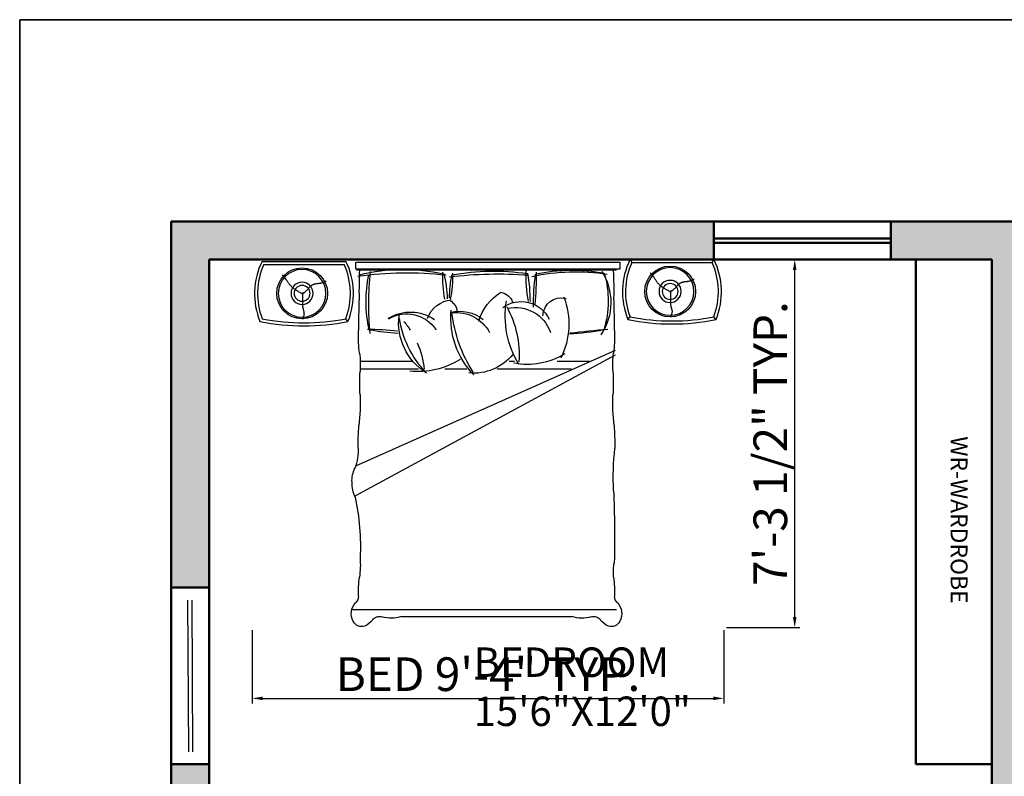
# Model space of a CAD drawing. Units: inches. Extents: x 1986 to 21484, y -1816 to 2016.
# Tile 44 of 85: x 2500 to 2734, y 1721 to 1901. Entities that reach past the tile are written whole.
import ezdxf

# ---------------------------------------------------------------- set-up
doc = ezdxf.new("R2010")
doc.units = ezdxf.units.IN
for name, color, linetype, lineweight in [('A-ANNO-DIMS', 2, 'Continuous', 18), ('A-ANNO-TEXT', 7, 'Continuous', 18), ('A-AREA-IDEN', 3, 'Continuous', 18), ('A-FURN', 8, 'Continuous', 18), ('A-GLAZ', 4, 'Continuous', 25), ('A-WALL', 7, 'Continuous', 50), ('A-WALL-PATT', 8, 'Continuous', 13), ('C-PROP', 7, 'Continuous', 35)]:
    doc.layers.add(name, color=color, linetype=linetype, lineweight=lineweight)
doc.layers.add('TEFRİŞ', color=11, linetype='Continuous')
doc.styles.get("Standard").update_dxf_attribs({"font": 'arial.ttf'})
doc.dimstyles.new('ISO-25', dxfattribs={"dimtxt": 8, "dimasz": 2.5, "dimexe": 1.25, "dimexo": 0.625, "dimtad": 1, "dimdec": 1, "dimlunit": 3, "dimtxsty": 'Standard', "dimcen": 2.5, "dimadec": 0, "dimazin": 0, "dimtfac": 1, "dimtdec": 1, "dimtmove": 0, "dimatfit": 3, "dimfxl": 1, "dimarcsym": 0})

# ---------------------------------------------------------------- blocks, each defined once
blk = doc.blocks.new('BED')
at = {"layer": 'TEFRİŞ'}
for p, q in [((2114.88, 1835.66), (2129.12, 1835.66)), ((2115.2, 1835.15), (2128.8, 1835.15)), ((2130.81, 1834.34), (2130.81, 1835.55)), ((2130.91, 1835.55), (2175.56, 1835.55)), ((2175.56, 1835.55), (2175.56, 1834.34)), ((2177.29, 1835.98), (2177.61, 1835.47)), ((2177.29, 1835.98), (2191.52, 1835.98)), ((2177.61, 1835.47), (2191.2, 1835.47)), ((2191.2, 1835.47), (2191.52, 1835.98)), ((2175.56, 1834.34), (2130.81, 1834.34)), ((2175, 1834.19), (2130.91, 1834.19)), ((2180.9, 1833.52), (2180.75, 1833.7)), ((2180.9, 1833.52), (2180.75, 1833.7)), ((2181.04, 1833.35), (2180.9, 1833.52)), ((2181.04, 1833.35), (2180.9, 1833.52)), ((2118.49, 1833.2), (2118.34, 1833.38)), ((2118.49, 1833.2), (2118.34, 1833.38)), ((2118.63, 1833.03), (2118.49, 1833.2)), ((2118.63, 1833.03), (2118.49, 1833.2)), ((2118.75, 1832.88), (2118.63, 1833.03)), ((2118.75, 1832.88), (2118.63, 1833.03)), ((2118.86, 1832.74), (2118.75, 1832.88)), ((2118.86, 1832.74), (2118.75, 1832.88)), ((2118.95, 1832.61), (2118.86, 1832.74)), ((2118.95, 1832.61), (2118.86, 1832.74)), ((2119.04, 1832.48), (2118.95, 1832.61)), ((2119.04, 1832.48), (2118.95, 1832.61)), ((2119.12, 1832.37), (2119.04, 1832.48)), ((2119.12, 1832.37), (2119.04, 1832.48)), ((2119.19, 1832.26), (2119.12, 1832.37)), ((2119.19, 1832.26), (2119.12, 1832.37)), ((2119.26, 1832.16), (2119.19, 1832.26)), ((2119.26, 1832.16), (2119.19, 1832.26)), ((2119.32, 1832.06), (2119.26, 1832.16)), ((2119.32, 1832.06), (2119.26, 1832.16)), ((2119.39, 1831.97), (2119.32, 1832.06)), ((2119.39, 1831.97), (2119.32, 1832.06)), ((2119.45, 1831.89), (2119.39, 1831.97)), ((2119.45, 1831.89), (2119.39, 1831.97)), ((2119.51, 1831.81), (2119.45, 1831.89)), ((2119.51, 1831.81), (2119.45, 1831.89)), ((2119.57, 1831.73), (2119.51, 1831.81)), ((2119.57, 1831.73), (2119.51, 1831.81)), ((2123.55, 1831.74), (2123.62, 1831.77)), ((2123.55, 1831.74), (2123.62, 1831.77)), ((2123.62, 1831.77), (2123.69, 1831.8)), ((2123.62, 1831.77), (2123.69, 1831.8)), ((2123.69, 1831.8), (2123.77, 1831.82)), ((2123.69, 1831.8), (2123.77, 1831.82)), ((2123.77, 1831.82), (2123.84, 1831.84)), ((2123.77, 1831.82), (2123.84, 1831.84)), ((2123.84, 1831.84), (2123.91, 1831.86)), ((2123.84, 1831.84), (2123.91, 1831.86)), ((2123.91, 1831.86), (2123.98, 1831.87)), ((2123.91, 1831.86), (2123.98, 1831.87)), ((2123.98, 1831.87), (2124.06, 1831.89)), ((2123.98, 1831.87), (2124.06, 1831.89)), ((2124.06, 1831.89), (2124.13, 1831.9)), ((2124.06, 1831.89), (2124.13, 1831.9)), ((2124.13, 1831.9), (2124.2, 1831.91)), ((2124.13, 1831.9), (2124.2, 1831.91)), ((2124.2, 1831.91), (2124.27, 1831.91)), ((2124.2, 1831.91), (2124.27, 1831.91)), ((2124.27, 1831.91), (2124.35, 1831.92)), ((2124.27, 1831.91), (2124.35, 1831.92)), ((2124.35, 1831.92), (2124.42, 1831.93)), ((2124.35, 1831.92), (2124.42, 1831.93)), ((2124.42, 1831.93), (2124.49, 1831.94)), ((2124.42, 1831.93), (2124.49, 1831.94)), ((2124.49, 1831.94), (2124.56, 1831.95)), ((2124.49, 1831.94), (2124.56, 1831.95)), ((2124.56, 1831.95), (2124.64, 1831.96)), ((2124.56, 1831.95), (2124.64, 1831.96)), ((2124.64, 1831.96), (2124.71, 1831.98)), ((2124.64, 1831.96), (2124.71, 1831.98)), ((2124.71, 1831.98), (2124.79, 1831.99)), ((2124.71, 1831.98), (2124.79, 1831.99)), ((2124.79, 1831.99), (2124.87, 1832.01)), ((2124.79, 1831.99), (2124.87, 1832.01)), ((2124.87, 1832.01), (2124.96, 1832.03)), ((2124.87, 1832.01), (2124.96, 1832.03)), ((2124.96, 1832.03), (2125.05, 1832.05)), ((2124.96, 1832.03), (2125.05, 1832.05)), ((2125.05, 1832.05), (2125.14, 1832.08)), ((2125.05, 1832.05), (2125.14, 1832.08)), ((2125.14, 1832.08), (2125.23, 1832.11)), ((2125.14, 1832.08), (2125.23, 1832.11)), ((2125.23, 1832.11), (2125.33, 1832.14)), ((2125.23, 1832.11), (2125.33, 1832.14)), ((2125.33, 1832.14), (2125.42, 1832.17)), ((2125.33, 1832.14), (2125.42, 1832.17)), ((2125.42, 1832.17), (2125.52, 1832.21)), ((2125.42, 1832.17), (2125.52, 1832.21)), ((2125.52, 1832.21), (2125.6, 1832.25)), ((2125.52, 1832.21), (2125.6, 1832.25)), ((2125.6, 1832.25), (2125.68, 1832.3)), ((2125.6, 1832.25), (2125.68, 1832.3)), ((2125.68, 1832.3), (2125.75, 1832.35)), ((2125.68, 1832.3), (2125.75, 1832.35)), ((2181.16, 1833.2), (2181.04, 1833.35)), ((2181.16, 1833.2), (2181.04, 1833.35)), ((2181.26, 1833.06), (2181.16, 1833.2)), ((2181.26, 1833.06), (2181.16, 1833.2)), ((2181.36, 1832.93), (2181.26, 1833.06)), ((2181.36, 1832.93), (2181.26, 1833.06)), ((2181.44, 1832.8), (2181.36, 1832.93)), ((2181.44, 1832.8), (2181.36, 1832.93)), ((2181.52, 1832.69), (2181.44, 1832.8)), ((2181.52, 1832.69), (2181.44, 1832.8)), ((2181.59, 1832.58), (2181.52, 1832.69)), ((2181.59, 1832.58), (2181.52, 1832.69)), ((2181.66, 1832.48), (2181.59, 1832.58)), ((2181.66, 1832.48), (2181.59, 1832.58)), ((2181.73, 1832.38), (2181.66, 1832.48)), ((2181.73, 1832.38), (2181.66, 1832.48)), ((2181.79, 1832.29), (2181.73, 1832.38)), ((2181.79, 1832.29), (2181.73, 1832.38)), ((2181.85, 1832.21), (2181.79, 1832.29)), ((2181.85, 1832.21), (2181.79, 1832.29)), ((2181.92, 1832.13), (2181.85, 1832.21)), ((2181.92, 1832.13), (2181.85, 1832.21)), ((2181.97, 1832.05), (2181.92, 1832.13)), ((2181.97, 1832.05), (2181.92, 1832.13)), ((2182.03, 1831.97), (2181.97, 1832.05)), ((2182.03, 1831.97), (2181.97, 1832.05)), ((2182.09, 1831.9), (2182.03, 1831.97)), ((2182.09, 1831.9), (2182.03, 1831.97)), ((2182.15, 1831.83), (2182.09, 1831.9)), ((2182.15, 1831.83), (2182.09, 1831.9)), ((2182.21, 1831.76), (2182.15, 1831.83)), ((2182.21, 1831.76), (2182.15, 1831.83)), ((2182.27, 1831.7), (2182.21, 1831.76)), ((2182.27, 1831.7), (2182.21, 1831.76)), ((2185.48, 1831.72), (2185.55, 1831.78)), ((2185.48, 1831.72), (2185.55, 1831.78)), ((2185.55, 1831.78), (2185.61, 1831.84)), ((2185.55, 1831.78), (2185.61, 1831.84)), ((2185.61, 1831.84), (2185.68, 1831.9)), ((2185.61, 1831.84), (2185.68, 1831.9)), ((2185.68, 1831.9), (2185.75, 1831.95)), ((2185.68, 1831.9), (2185.75, 1831.95)), ((2185.75, 1831.95), (2185.82, 1831.99)), ((2185.75, 1831.95), (2185.82, 1831.99)), ((2185.82, 1831.99), (2185.89, 1832.03)), ((2185.82, 1831.99), (2185.89, 1832.03)), ((2185.89, 1832.03), (2185.96, 1832.06)), ((2185.89, 1832.03), (2185.96, 1832.06)), ((2185.96, 1832.06), (2186.03, 1832.09)), ((2185.96, 1832.06), (2186.03, 1832.09)), ((2186.03, 1832.09), (2186.1, 1832.12)), ((2186.03, 1832.09), (2186.1, 1832.12)), ((2186.1, 1832.12), (2186.17, 1832.14)), ((2186.1, 1832.12), (2186.17, 1832.14)), ((2186.17, 1832.14), (2186.24, 1832.16)), ((2186.17, 1832.14), (2186.24, 1832.16)), ((2186.24, 1832.16), (2186.32, 1832.18)), ((2186.24, 1832.16), (2186.32, 1832.18)), ((2186.32, 1832.18), (2186.39, 1832.19)), ((2186.32, 1832.18), (2186.39, 1832.19)), ((2186.39, 1832.19), (2186.46, 1832.21)), ((2186.39, 1832.19), (2186.46, 1832.21)), ((2186.46, 1832.21), (2186.53, 1832.22)), ((2186.46, 1832.21), (2186.53, 1832.22)), ((2186.53, 1832.22), (2186.61, 1832.23)), ((2186.53, 1832.22), (2186.61, 1832.23)), ((2186.61, 1832.23), (2186.68, 1832.23)), ((2186.61, 1832.23), (2186.68, 1832.23)), ((2186.68, 1832.23), (2186.75, 1832.24)), ((2186.68, 1832.23), (2186.75, 1832.24)), ((2186.75, 1832.24), (2186.82, 1832.25)), ((2186.75, 1832.24), (2186.82, 1832.25)), ((2186.82, 1832.25), (2186.9, 1832.26)), ((2186.82, 1832.25), (2186.9, 1832.26)), ((2186.9, 1832.26), (2186.97, 1832.27)), ((2186.9, 1832.26), (2186.97, 1832.27)), ((2186.97, 1832.27), (2187.04, 1832.28)), ((2186.97, 1832.27), (2187.04, 1832.28)), ((2187.04, 1832.28), (2187.12, 1832.3)), ((2187.04, 1832.28), (2187.12, 1832.3)), ((2187.12, 1832.3), (2187.2, 1832.31)), ((2187.12, 1832.3), (2187.2, 1832.31)), ((2187.2, 1832.31), (2187.28, 1832.33)), ((2187.2, 1832.31), (2187.28, 1832.33)), ((2187.28, 1832.33), (2187.36, 1832.35)), ((2187.28, 1832.33), (2187.36, 1832.35)), ((2187.36, 1832.35), (2187.45, 1832.37)), ((2187.36, 1832.35), (2187.45, 1832.37)), ((2187.45, 1832.37), (2187.54, 1832.4)), ((2187.45, 1832.37), (2187.54, 1832.4)), ((2187.54, 1832.4), (2187.64, 1832.43)), ((2187.54, 1832.4), (2187.64, 1832.43)), ((2187.64, 1832.43), (2187.74, 1832.46)), ((2187.64, 1832.43), (2187.74, 1832.46)), ((2187.74, 1832.46), (2187.83, 1832.49)), ((2187.74, 1832.46), (2187.83, 1832.49)), ((2187.83, 1832.49), (2187.92, 1832.53)), ((2187.83, 1832.49), (2187.92, 1832.53)), ((2187.92, 1832.53), (2188.01, 1832.57)), ((2187.92, 1832.53), (2188.01, 1832.57)), ((2188.01, 1832.57), (2188.09, 1832.62)), ((2188.01, 1832.57), (2188.09, 1832.62)), ((2188.09, 1832.62), (2188.15, 1832.67)), ((2188.09, 1832.62), (2188.15, 1832.67)), ((2119.63, 1831.65), (2119.57, 1831.73)), ((2119.63, 1831.65), (2119.57, 1831.73)), ((2119.69, 1831.58), (2119.63, 1831.65)), ((2119.69, 1831.58), (2119.63, 1831.65)), ((2119.75, 1831.51), (2119.69, 1831.58)), ((2119.75, 1831.51), (2119.69, 1831.58)), ((2119.81, 1831.44), (2119.75, 1831.51)), ((2119.81, 1831.44), (2119.75, 1831.51)), ((2119.87, 1831.38), (2119.81, 1831.44)), ((2119.87, 1831.38), (2119.81, 1831.44)), ((2119.93, 1831.31), (2119.87, 1831.38)), ((2119.93, 1831.31), (2119.87, 1831.38)), ((2119.99, 1831.25), (2119.93, 1831.31)), ((2119.99, 1831.25), (2119.93, 1831.31)), ((2120.05, 1831.2), (2119.99, 1831.25)), ((2120.05, 1831.2), (2119.99, 1831.25)), ((2120.12, 1831.14), (2120.05, 1831.2)), ((2120.12, 1831.14), (2120.05, 1831.2)), ((2120.18, 1831.09), (2120.12, 1831.14)), ((2120.18, 1831.09), (2120.12, 1831.14)), ((2120.25, 1831.04), (2120.18, 1831.09)), ((2120.25, 1831.04), (2120.18, 1831.09)), ((2120.32, 1830.99), (2120.25, 1831.04)), ((2120.32, 1830.99), (2120.25, 1831.04)), ((2120.39, 1830.94), (2120.32, 1830.99)), ((2120.39, 1830.94), (2120.32, 1830.99)), ((2120.47, 1830.9), (2120.39, 1830.94)), ((2120.47, 1830.9), (2120.39, 1830.94)), ((2120.54, 1830.85), (2120.47, 1830.9)), ((2120.54, 1830.85), (2120.47, 1830.9)), ((2120.62, 1830.8), (2120.54, 1830.85)), ((2120.62, 1830.8), (2120.54, 1830.85)), ((2120.7, 1830.75), (2120.62, 1830.8)), ((2120.7, 1830.75), (2120.62, 1830.8)), ((2120.79, 1830.7), (2120.7, 1830.75)), ((2120.79, 1830.7), (2120.7, 1830.75)), ((2120.88, 1830.65), (2120.79, 1830.7)), ((2120.88, 1830.65), (2120.79, 1830.7)), ((2120.98, 1830.59), (2120.88, 1830.65)), ((2120.98, 1830.59), (2120.88, 1830.65)), ((2121.09, 1830.52), (2120.98, 1830.59)), ((2121.09, 1830.52), (2120.98, 1830.59)), ((2121.21, 1830.45), (2121.09, 1830.52)), ((2121.21, 1830.45), (2121.09, 1830.52)), ((2121.34, 1830.38), (2121.21, 1830.45)), ((2121.34, 1830.38), (2121.21, 1830.45)), ((2121.49, 1830.29), (2121.34, 1830.38)), ((2121.49, 1830.29), (2121.34, 1830.38)), ((2121.66, 1830.21), (2121.49, 1830.29)), ((2121.66, 1830.21), (2121.49, 1830.29)), ((2121.66, 1830.18), (2121.87, 1830.29)), ((2121.66, 1830.18), (2121.87, 1830.29)), ((2121.85, 1830.11), (2121.66, 1830.21)), ((2121.85, 1830.11), (2121.66, 1830.21)), ((2121.76, 1830.38), (2121.74, 1830.17)), ((2121.76, 1830.38), (2121.74, 1830.17)), ((2121.74, 1830.17), (2121.74, 1829.99)), ((2121.74, 1830.17), (2121.74, 1829.99)), ((2121.87, 1830.29), (2122.04, 1830.4)), ((2121.87, 1830.29), (2122.04, 1830.4)), ((2122.04, 1830.4), (2122.2, 1830.51)), ((2122.04, 1830.4), (2122.2, 1830.51)), ((2122.2, 1830.51), (2122.33, 1830.61)), ((2122.2, 1830.51), (2122.33, 1830.61)), ((2122.33, 1830.61), (2122.45, 1830.72)), ((2122.33, 1830.61), (2122.45, 1830.72)), ((2122.45, 1830.72), (2122.55, 1830.82)), ((2122.45, 1830.72), (2122.55, 1830.82)), ((2122.55, 1830.82), (2122.64, 1830.91)), ((2122.55, 1830.82), (2122.64, 1830.91)), ((2122.64, 1830.91), (2122.72, 1831.01)), ((2122.64, 1830.91), (2122.72, 1831.01)), ((2122.72, 1831.01), (2122.8, 1831.09)), ((2122.72, 1831.01), (2122.8, 1831.09)), ((2122.8, 1831.09), (2122.87, 1831.18)), ((2122.8, 1831.09), (2122.87, 1831.18)), ((2122.87, 1831.18), (2122.94, 1831.26)), ((2122.87, 1831.18), (2122.94, 1831.26)), ((2122.94, 1831.26), (2123.01, 1831.33)), ((2122.94, 1831.26), (2123.01, 1831.33)), ((2123.01, 1831.33), (2123.08, 1831.4)), ((2123.01, 1831.33), (2123.08, 1831.4)), ((2123.08, 1831.4), (2123.14, 1831.46)), ((2123.08, 1831.4), (2123.14, 1831.46)), ((2123.14, 1831.46), (2123.21, 1831.52)), ((2123.14, 1831.46), (2123.21, 1831.52)), ((2123.21, 1831.52), (2123.27, 1831.58)), ((2123.21, 1831.52), (2123.27, 1831.58)), ((2123.27, 1831.58), (2123.34, 1831.63)), ((2123.27, 1831.58), (2123.34, 1831.63)), ((2123.34, 1831.63), (2123.41, 1831.67)), ((2123.34, 1831.63), (2123.41, 1831.67)), ((2123.41, 1831.67), (2123.48, 1831.71)), ((2123.41, 1831.67), (2123.48, 1831.71)), ((2123.48, 1831.71), (2123.55, 1831.74)), ((2123.48, 1831.71), (2123.55, 1831.74)), ((2182.33, 1831.63), (2182.27, 1831.7)), ((2182.33, 1831.63), (2182.27, 1831.7)), ((2182.4, 1831.57), (2182.33, 1831.63)), ((2182.4, 1831.57), (2182.33, 1831.63)), ((2182.46, 1831.52), (2182.4, 1831.57)), ((2182.46, 1831.52), (2182.4, 1831.57)), ((2182.52, 1831.46), (2182.46, 1831.52)), ((2182.52, 1831.46), (2182.46, 1831.52)), ((2182.59, 1831.41), (2182.52, 1831.46)), ((2182.59, 1831.41), (2182.52, 1831.46)), ((2182.66, 1831.36), (2182.59, 1831.41)), ((2182.66, 1831.36), (2182.59, 1831.41)), ((2182.73, 1831.31), (2182.66, 1831.36)), ((2182.73, 1831.31), (2182.66, 1831.36)), ((2182.8, 1831.26), (2182.73, 1831.31)), ((2182.8, 1831.26), (2182.73, 1831.31)), ((2182.87, 1831.22), (2182.8, 1831.26)), ((2182.87, 1831.22), (2182.8, 1831.26)), ((2182.95, 1831.17), (2182.87, 1831.22)), ((2182.95, 1831.17), (2182.87, 1831.22)), ((2183.03, 1831.12), (2182.95, 1831.17)), ((2183.03, 1831.12), (2182.95, 1831.17)), ((2183.11, 1831.07), (2183.03, 1831.12)), ((2183.11, 1831.07), (2183.03, 1831.12)), ((2183.2, 1831.02), (2183.11, 1831.07)), ((2183.2, 1831.02), (2183.11, 1831.07)), ((2183.29, 1830.97), (2183.2, 1831.02)), ((2183.29, 1830.97), (2183.2, 1831.02)), ((2183.39, 1830.91), (2183.29, 1830.97)), ((2183.39, 1830.91), (2183.29, 1830.97)), ((2183.49, 1830.84), (2183.39, 1830.91)), ((2183.49, 1830.84), (2183.39, 1830.91)), ((2183.61, 1830.77), (2183.49, 1830.84)), ((2183.61, 1830.77), (2183.49, 1830.84)), ((2183.75, 1830.7), (2183.61, 1830.77)), ((2183.75, 1830.7), (2183.61, 1830.77)), ((2183.9, 1830.61), (2183.75, 1830.7)), ((2183.9, 1830.61), (2183.75, 1830.7)), ((2184.06, 1830.53), (2183.9, 1830.61)), ((2184.06, 1830.53), (2183.9, 1830.61)), ((2184.25, 1830.43), (2184.06, 1830.53)), ((2184.25, 1830.43), (2184.06, 1830.53)), ((2184.07, 1830.5), (2184.27, 1830.61)), ((2184.07, 1830.5), (2184.27, 1830.61)), ((2184.15, 1830.49), (2184.14, 1830.31)), ((2184.15, 1830.49), (2184.14, 1830.31)), ((2184.14, 1830.31), (2184.14, 1830.15)), ((2184.14, 1830.31), (2184.14, 1830.15)), ((2184.14, 1830.15), (2184.14, 1830.01)), ((2184.14, 1830.15), (2184.14, 1830.01)), ((2184.17, 1830.7), (2184.15, 1830.49)), ((2184.17, 1830.7), (2184.15, 1830.49)), ((2184.27, 1830.61), (2184.45, 1830.72)), ((2184.27, 1830.61), (2184.45, 1830.72)), ((2184.45, 1830.72), (2184.6, 1830.83)), ((2184.45, 1830.72), (2184.6, 1830.83)), ((2184.6, 1830.83), (2184.74, 1830.93)), ((2184.6, 1830.83), (2184.74, 1830.93)), ((2184.74, 1830.93), (2184.85, 1831.04)), ((2184.74, 1830.93), (2184.85, 1831.04)), ((2184.85, 1831.04), (2184.95, 1831.14)), ((2184.85, 1831.04), (2184.95, 1831.14)), ((2184.95, 1831.14), (2185.05, 1831.23)), ((2184.95, 1831.14), (2185.05, 1831.23)), ((2185.05, 1831.23), (2185.13, 1831.33)), ((2185.05, 1831.23), (2185.13, 1831.33)), ((2185.13, 1831.33), (2185.21, 1831.41)), ((2185.13, 1831.33), (2185.21, 1831.41)), ((2185.21, 1831.41), (2185.28, 1831.5)), ((2185.21, 1831.41), (2185.28, 1831.5)), ((2185.28, 1831.5), (2185.35, 1831.58)), ((2185.28, 1831.5), (2185.35, 1831.58)), ((2185.35, 1831.58), (2185.42, 1831.65)), ((2185.35, 1831.58), (2185.42, 1831.65)), ((2185.42, 1831.65), (2185.48, 1831.72)), ((2185.42, 1831.65), (2185.48, 1831.72)), ((2121.74, 1829.99), (2121.73, 1829.83)), ((2121.74, 1829.99), (2121.73, 1829.83)), ((2121.73, 1829.83), (2121.73, 1829.69)), ((2121.73, 1829.83), (2121.73, 1829.69)), ((2121.73, 1829.69), (2121.73, 1829.57)), ((2121.73, 1829.69), (2121.73, 1829.57)), ((2121.73, 1829.57), (2121.73, 1829.45)), ((2121.73, 1829.57), (2121.73, 1829.45)), ((2121.73, 1829.45), (2121.74, 1829.35)), ((2121.73, 1829.45), (2121.74, 1829.35)), ((2121.74, 1828.89), (2121.73, 1828.8)), ((2121.74, 1828.89), (2121.73, 1828.8)), ((2121.73, 1828.8), (2121.73, 1828.72)), ((2121.73, 1828.8), (2121.73, 1828.72)), ((2121.73, 1828.72), (2121.73, 1828.64)), ((2121.73, 1828.72), (2121.73, 1828.64)), ((2121.73, 1828.64), (2121.73, 1828.56)), ((2121.73, 1828.64), (2121.73, 1828.56)), ((2121.73, 1828.56), (2121.73, 1828.48)), ((2121.73, 1828.56), (2121.73, 1828.48)), ((2121.73, 1828.48), (2121.73, 1828.4)), ((2121.73, 1828.48), (2121.73, 1828.4)), ((2121.74, 1829.35), (2121.74, 1829.25)), ((2121.74, 1829.35), (2121.74, 1829.25)), ((2121.74, 1829.25), (2121.74, 1829.16)), ((2121.74, 1829.25), (2121.74, 1829.16)), ((2121.74, 1829.16), (2121.74, 1829.06)), ((2121.74, 1829.16), (2121.74, 1829.06)), ((2121.74, 1829.06), (2121.74, 1828.97)), ((2121.74, 1829.06), (2121.74, 1828.97)), ((2121.74, 1828.97), (2121.74, 1828.89)), ((2121.74, 1828.97), (2121.74, 1828.89)), ((2184.14, 1829.04), (2184.13, 1828.96)), ((2184.14, 1829.04), (2184.13, 1828.96)), ((2184.13, 1828.96), (2184.13, 1828.88)), ((2184.13, 1828.96), (2184.13, 1828.88)), ((2184.13, 1828.88), (2184.13, 1828.8)), ((2184.13, 1828.88), (2184.13, 1828.8)), ((2184.13, 1828.8), (2184.14, 1828.72)), ((2184.13, 1828.8), (2184.14, 1828.72)), ((2184.14, 1830.01), (2184.14, 1829.89)), ((2184.14, 1830.01), (2184.14, 1829.89)), ((2184.14, 1829.89), (2184.14, 1829.77)), ((2184.14, 1829.89), (2184.14, 1829.77)), ((2184.14, 1829.77), (2184.14, 1829.67)), ((2184.14, 1829.77), (2184.14, 1829.67)), ((2184.14, 1829.67), (2184.15, 1829.57)), ((2184.14, 1829.67), (2184.15, 1829.57)), ((2184.15, 1829.38), (2184.14, 1829.29)), ((2184.15, 1829.38), (2184.14, 1829.29)), ((2184.14, 1829.29), (2184.14, 1829.21)), ((2184.14, 1829.29), (2184.14, 1829.21)), ((2184.14, 1829.21), (2184.14, 1829.12)), ((2184.14, 1829.21), (2184.14, 1829.12)), ((2184.14, 1829.12), (2184.14, 1829.04)), ((2184.14, 1829.12), (2184.14, 1829.04)), ((2184.14, 1828.72), (2184.14, 1828.65)), ((2184.14, 1828.72), (2184.14, 1828.65)), ((2184.14, 1828.65), (2184.15, 1828.57)), ((2184.14, 1828.65), (2184.15, 1828.57)), ((2184.15, 1829.57), (2184.15, 1829.48)), ((2184.15, 1829.57), (2184.15, 1829.48)), ((2184.15, 1829.48), (2184.15, 1829.38)), ((2184.15, 1829.48), (2184.15, 1829.38)), ((2184.15, 1828.57), (2184.15, 1828.5)), ((2184.15, 1828.57), (2184.15, 1828.5)), ((2184.15, 1828.5), (2184.16, 1828.42)), ((2184.15, 1828.5), (2184.16, 1828.42)), ((2184.16, 1828.42), (2184.17, 1828.35)), ((2184.16, 1828.42), (2184.17, 1828.35)), ((2121.73, 1828.4), (2121.73, 1828.33)), ((2121.73, 1828.4), (2121.73, 1828.33)), ((2121.73, 1828.33), (2121.74, 1828.25)), ((2121.73, 1828.33), (2121.74, 1828.25)), ((2121.74, 1828.25), (2121.75, 1828.18)), ((2121.74, 1828.25), (2121.75, 1828.18)), ((2121.75, 1828.18), (2121.75, 1828.1)), ((2121.75, 1828.18), (2121.75, 1828.1)), ((2121.75, 1828.1), (2121.76, 1828.03)), ((2121.75, 1828.1), (2121.76, 1828.03)), ((2121.76, 1828.03), (2121.78, 1827.95)), ((2121.76, 1828.03), (2121.78, 1827.95)), ((2121.78, 1827.95), (2121.79, 1827.88)), ((2121.78, 1827.95), (2121.79, 1827.88)), ((2121.79, 1827.88), (2121.8, 1827.8)), ((2121.79, 1827.88), (2121.8, 1827.8)), ((2121.8, 1827.8), (2121.82, 1827.72)), ((2121.8, 1827.8), (2121.82, 1827.72)), ((2121.82, 1827.72), (2121.84, 1827.65)), ((2121.82, 1827.72), (2121.84, 1827.65)), ((2121.84, 1827.65), (2121.85, 1827.57)), ((2121.84, 1827.65), (2121.85, 1827.57)), ((2121.85, 1827.57), (2121.87, 1827.49)), ((2121.85, 1827.57), (2121.87, 1827.49)), ((2121.87, 1827.49), (2121.89, 1827.41)), ((2121.87, 1827.49), (2121.89, 1827.41)), ((2121.89, 1827.41), (2121.91, 1827.33)), ((2121.89, 1827.41), (2121.91, 1827.33)), ((2121.91, 1827.33), (2121.93, 1827.26)), ((2121.91, 1827.33), (2121.93, 1827.26)), ((2121.93, 1827.26), (2121.95, 1827.18)), ((2121.93, 1827.26), (2121.95, 1827.18)), ((2121.95, 1827.18), (2121.97, 1827.09)), ((2121.95, 1827.18), (2121.97, 1827.09)), ((2121.97, 1827.09), (2121.99, 1827.01)), ((2121.97, 1827.09), (2121.99, 1827.01)), ((2121.99, 1827.01), (2122, 1826.93)), ((2121.99, 1827.01), (2122, 1826.93)), ((2122, 1826.74), (2121.99, 1826.64)), ((2122, 1826.74), (2121.99, 1826.64)), ((2122, 1826.93), (2122.01, 1826.84)), ((2122, 1826.93), (2122.01, 1826.84)), ((2122.01, 1826.84), (2122, 1826.74)), ((2122.01, 1826.84), (2122, 1826.74)), ((2184.17, 1828.35), (2184.18, 1828.27)), ((2184.17, 1828.35), (2184.18, 1828.27)), ((2184.18, 1828.27), (2184.19, 1828.2)), ((2184.18, 1828.27), (2184.19, 1828.2)), ((2184.19, 1828.2), (2184.21, 1828.12)), ((2184.19, 1828.2), (2184.21, 1828.12)), ((2184.21, 1828.12), (2184.22, 1828.04)), ((2184.21, 1828.12), (2184.22, 1828.04)), ((2184.22, 1828.04), (2184.24, 1827.97)), ((2184.22, 1828.04), (2184.24, 1827.97)), ((2184.24, 1827.97), (2184.26, 1827.89)), ((2184.24, 1827.97), (2184.26, 1827.89)), ((2184.26, 1827.89), (2184.28, 1827.81)), ((2184.26, 1827.89), (2184.28, 1827.81)), ((2184.28, 1827.81), (2184.3, 1827.73)), ((2184.28, 1827.81), (2184.3, 1827.73)), ((2184.3, 1827.73), (2184.32, 1827.65)), ((2184.3, 1827.73), (2184.32, 1827.65)), ((2184.32, 1827.65), (2184.34, 1827.58)), ((2184.32, 1827.65), (2184.34, 1827.58)), ((2184.35, 1826.74), (2184.32, 1826.63)), ((2184.35, 1826.74), (2184.32, 1826.63)), ((2184.34, 1827.58), (2184.36, 1827.5)), ((2184.34, 1827.58), (2184.36, 1827.5)), ((2184.38, 1826.86), (2184.35, 1826.74)), ((2184.38, 1826.86), (2184.35, 1826.74)), ((2184.36, 1827.5), (2184.38, 1827.41)), ((2184.36, 1827.5), (2184.38, 1827.41)), ((2184.38, 1827.41), (2184.4, 1827.33)), ((2184.38, 1827.41), (2184.4, 1827.33)), ((2184.4, 1826.96), (2184.38, 1826.86)), ((2184.4, 1826.96), (2184.38, 1826.86)), ((2184.4, 1827.33), (2184.41, 1827.25)), ((2184.4, 1827.33), (2184.41, 1827.25)), ((2184.41, 1827.06), (2184.4, 1826.96)), ((2184.41, 1827.06), (2184.4, 1826.96)), ((2184.41, 1827.25), (2184.41, 1827.16)), ((2184.41, 1827.25), (2184.41, 1827.16)), ((2184.41, 1827.16), (2184.41, 1827.06)), ((2184.41, 1827.16), (2184.41, 1827.06)), ((2121.78, 1825.93), (2121.74, 1825.8)), ((2121.78, 1825.93), (2121.74, 1825.8)), ((2121.83, 1826.06), (2121.78, 1825.93)), ((2121.83, 1826.06), (2121.78, 1825.93)), ((2121.87, 1826.19), (2121.83, 1826.06)), ((2121.87, 1826.19), (2121.83, 1826.06)), ((2121.91, 1826.31), (2121.87, 1826.19)), ((2121.91, 1826.31), (2121.87, 1826.19)), ((2121.95, 1826.42), (2121.91, 1826.31)), ((2121.95, 1826.42), (2121.91, 1826.31)), ((2121.97, 1826.54), (2121.95, 1826.42)), ((2121.97, 1826.54), (2121.95, 1826.42)), ((2121.99, 1826.64), (2121.97, 1826.54)), ((2121.99, 1826.64), (2121.97, 1826.54)), ((2129.46, 1825.49), (2129.09, 1825.93)), ((2176.94, 1825.81), (2177.31, 1826.25)), ((2184.19, 1826.25), (2184.14, 1826.12)), ((2184.19, 1826.25), (2184.14, 1826.12)), ((2184.23, 1826.38), (2184.19, 1826.25)), ((2184.23, 1826.38), (2184.19, 1826.25)), ((2184.28, 1826.51), (2184.23, 1826.38)), ((2184.28, 1826.51), (2184.23, 1826.38)), ((2184.32, 1826.63), (2184.28, 1826.51)), ((2184.32, 1826.63), (2184.28, 1826.51)), ((2191.87, 1825.81), (2191.5, 1826.25)), ((2174.77, 1820.53), (2130.76, 1800.91)), ((2174.77, 1819.77), (2130.6, 1795.83)), ((2140.43, 1818.69), (2131.53, 1818.69)), ((2157.71, 1818.69), (2156.77, 1818.69)), ((2170.41, 1818.69), (2164.92, 1818.69)), ((2141.43, 1817.4), (2131.53, 1817.4)), ((2149.62, 1817.4), (2145.88, 1817.4)), ((2167.36, 1817.4), (2154.77, 1817.4)), ((2175, 1776.57), (2130.11, 1776.57)), ((2138.52, 1775.41), (2167.39, 1775.41))]:
    blk.add_line(p, q, dxfattribs=at)
for centre, radius, start, end in [((2126, 1830.19), 12.39, 153.8162, 202.314), ((2126, 1830.19), 11.88, 155.3335, 201.0157), ((2118, 1830.19), 11.88, 338.9843, 24.6665), ((2118, 1830.19), 12.39, 337.686, 26.1838), ((2188.4, 1830.51), 12.39, 153.8162, 202.314), ((2188.4, 1830.51), 11.88, 155.3335, 201.0157), ((2180.41, 1830.51), 11.88, 338.9843, 24.6665), ((2180.41, 1830.51), 12.39, 337.686, 26.1838), ((2122, 1861.35), 36.63, 258.2443, 281.7557), ((2122, 1861.35), 36.12, 258.6773, 281.3227), ((2184.41, 1861.67), 36.63, 258.2443, 281.7557), ((2184.41, 1861.67), 36.12, 258.6773, 281.3227)]:
    blk.add_arc(centre, radius, start, end, dxfattribs=at)
at = {"layer": 'TEFRİŞ', "extrusion": (0, 0, -1)}
for centre, major_axis, ratio, start_param, end_param in [((2121.68, 1830.24), (-3.05, -3.05), 1, 3.926991, 10.210176), ((2121.68, 1830.24), (2.86, -2.86), 1, 5.497787, 11.780972), ((2121.68, 1830.24), (2.86, -2.86), 1, 5.497787, 11.780972), ((2139.43, 1773.84), (-42.35, 42.35), 1, 0.646251, 0.896949), ((2206.14, 1830.73), (-52.86, -52.86), 1, 0.767743, 0.83177), ((2138.85, 1803.05), (-22.1, 22.1), 1, 0.544604, 1.006234), ((2181.61, 1828.44), (-34.39, 34.39), 1, -0.888486, -0.672463), ((2164.51, 1832.79), (-13.41, 13.41), 1, -0.974476, -0.730892), ((2127.6, 1828.81), (-13.23, 13.23), 1, 2.100388, 2.328052), ((2155, 1761.9), (-50.65, -50.65), 1, 2.239512, 2.426533), ((2128.44, 1832.96), (-13.26, -13.26), 1, 3.889049, 4.127298), ((2154.12, 1796.61), (-26.46, 26.46), 1, 0.596409, 0.940188), ((2183.72, 1833.22), (-17, 17), 1, -0.967105, -0.749712), ((2134, 1828.8), (-18.62, 18.62), 1, 2.173461, 2.355043), ((2168.35, 1789.27), (-1.33, 44.62), 0.875277, -0.163954, 0.163954), ((2199.2, 1828.45), (-27.06, -27.06), 1, 0.770625, 0.917228), ((2087.32, 1833.96), (-52.37, 52.37), 1, 2.358049, 2.431787), ((2167.6, 1797.72), (-0.51, 36.47), 0.865194, -0.185965, 0.185965), ((2164.15, 1828.7), (-6.99, 6.99), 1, 1.789136, 2.946702), ((2156.76, 1828.98), (-11.9, -11.9), 1, 3.646453, 4.226155), ((2099.77, 1830.73), (-52.86, 52.86), 1, 2.311571, 2.373849), ((2184.09, 1830.56), (-3.05, -3.05), 1, 3.926991, 10.210176), ((2184.09, 1830.56), (2.86, -2.86), 1, 5.497787, 11.780972), ((2184.09, 1830.56), (2.86, -2.86), 1, 5.497787, 11.780972), ((2121.68, 1830.24), (1.33, -1.33), 1, 5.497787, 11.780972), ((2121.68, 1830.24), (1.33, -1.33), 1, 5.497787, 11.780972), ((2154.7, 1828.89), (-15.68, 15.68), 1, -1.00675, -0.580436), ((2172.01, 1828.66), (-17.93, 17.93), 1, -0.753394, -0.598744), ((2184.09, 1830.56), (1.33, -1.33), 1, 5.497787, 11.780972), ((2184.09, 1830.56), (1.33, -1.33), 1, 5.497787, 11.780972), ((2184.09, 1830.56), (0.952, -0.952), 1, 5.497787, 11.780972), ((2184.09, 1830.56), (0.952, -0.952), 1, 5.497787, 11.780972), ((2121.68, 1830.24), (0.952, -0.952), 1, 5.497787, 11.780972), ((2121.68, 1830.24), (0.952, -0.952), 1, 5.497787, 11.780972), ((2159.55, 1823.33), (-5.81, 5.81), 1, -0.516587, 0.256776), ((2154.84, 1827.75), (-1.93, 1.93), 1, 0.997904, 1.977819), ((2675.38, 1815.09), (-384.79, -384.79), 1, 0.80103, 0.811711), ((2147.44, 1824.41), (-3.36, -3.36), 1, 1.11934, 2.270556), ((2145.66, 1827.01), (-1.62, 1.62), 1, 1.310976, 2.284591), ((2172, 1826.44), (-11.23, 11.23), 1, -1.332486, -0.624868), ((2158.82, 1823.55), (-3.74, -3.74), 1, 1.730792, 3.47045), ((2166.67, 1824.96), (-2.93, 3.91), 0.760601, -0.723751, 0.723751), ((2153.88, 1825.05), (-9.22, 9.22), 1, 1.994956, 2.818753), ((1630.53, 1815.09), (-384.79, 384.79), 1, 2.329881, 2.340562), ((2140.05, 1819.86), (-5.1, 5.1), 1, 0.238357, 1.390139), ((2139.42, 1820.79), (-4.21, -4.21), 1, 1.82161, 3.349145), ((2160.6, 1825.98), (-9.68, -9.68), 1, 0.009196, 0.886853), ((2148.35, 1820.65), (-4.63, -4.63), 1, 2.117602, 3.020837), ((2147.86, 1820.64), (-4.48, 4.48), 1, 0.665914, 1.867503), ((2170.68, 1829.67), (-16.79, 16.79), 1, -1.354718, -0.902276), ((2141.71, 1819.83), (-11.86, 11.86), 1, 1.850844, 2.42862), ((2157.83, 1821.53), (-4.47, 4.47), 1, 0.576679, 2.021689), ((2148.15, 1825.25), (-7.14, -7.14), 1, 6.061986, 7.190757), ((2154.93, 1828.48), (-11.96, 11.96), 1, -1.530302, -0.934407), ((2127.37, 1815.76), (-10.68, 10.68), 1, 1.657204, 1.779381), ((2146.08, 1822.57), (-10.5, 10.5), 1, -0.951783, -0.716225), ((2132.43, 1774.09), (-35.41, -35.41), 1, 2.362911, 2.464592), ((2140.17, 1862.96), (-27.99, 27.99), 1, 3.983025, 4.107469), ((2165.73, 1860.69), (-26.41, -26.41), 1, 5.306413, 5.463767), ((2199.62, 1529.47), (-209.2, 209.2), 1, 0.675361, 0.697001), ((2159.82, 1822.57), (-10.5, -10.5), 1, 3.857817, 4.093375), ((2127.37, 1815.76), (-10.68, 10.68), 1, 1.94252, 2.248924), ((2111.06, 1818.12), (-14.48, 14.48), 1, 2.258605, 2.412359), ((2194.85, 1818.12), (-14.48, 14.48), 1, -0.841563, -0.687809), ((2141.33, 1830.48), (-9.55, -9.55), 1, 4.941413, 5.601673), ((2150.79, 1825.18), (-6, 6), 1, 3.032122, 4.026148), ((2159.02, 1834.9), (-3.04, 16.53), 0.830169, 2.822117, 3.461068), ((2169.92, 1815.01), (-27.2, -27.2), 1, 0.734393, 0.836404), ((2135.98, 1815.01), (-27.2, -27.2), 1, 3.875985, 3.977996), ((2098.24, 1811.68), (-23.54, -23.54), 1, 3.885834, 4.043401), ((2207.66, 1811.68), (-23.54, -23.54), 1, 0.668988, 0.826555), ((2189.03, 1803.74), (-40.91, -40.91), 1, 0.789771, 0.855756), ((2116.87, 1803.74), (-40.91, 40.91), 1, 2.285836, 2.351822), ((2122.14, 1803.63), (-6.39, -6.39), 1, 3.886359, 4.265474), ((2222.76, 1798.77), (-34.16, -34.16), 1, 0.743488, 0.893627), ((2135.02, 1798.41), (-3.45, 3.45), 1, -0.831635, -0.314979), ((2135.48, 1798), (-3.77, -3.77), 1, 0.329385, 0.820948), ((2148.06, 1790.38), (-0.75, 67.37), 0.394952, 1.480524, 1.661068), ((2127.76, 1790.23), (-1, 12.37), 0.296708, 1.141067, 2.000525), ((2118.49, 1784.2), (-9.24, -9.24), 1, 3.839645, 4.088086), ((2182.27, 1782.99), (-5.52, -5.52), 1, 0.671703, 0.993321), ((2162.12, 1778.86), (-21.85, 21.85), 1, -0.78611, -0.680117), ((2143.78, 1778.86), (-21.85, 21.85), 1, 2.250913, 2.356906), ((2129.83, 1778.8), (-0.986, 0.986), 1, 2.330985, 3.163296), ((2176.08, 1778.8), (-0.986, 0.986), 1, 4.690686, 5.522997), ((2132.72, 1775.92), (-1.91, -1.91), 1, 0.284117, 1.557111), ((2173.18, 1775.92), (-1.91, -1.91), 1, 3.155278, 4.428271), ((2134.73, 1774.06), (-0.964, -0.964), 1, 1.381176, 2.701227), ((2136.75, 1781.14), (-4.24, 4.24), 1, 3.62713, 4.188813), ((2169.16, 1781.14), (-4.24, 4.24), 1, 3.665169, 4.226852), ((2171.17, 1774.06), (-0.964, -0.964), 1, 2.011162, 3.331212), ((2131.79, 1775.28), (-1.11, 1.11), 1, 3.629269, 5.067473), ((2130.83, 1777), (-2.49, -2.49), 1, 4.590984, 5.084038), ((2175.07, 1777), (-2.49, 2.49), 1, 4.34074, 4.833793), ((2174.12, 1775.28), (-1.11, 1.11), 1, 2.786508, 4.224712)]:
    blk.add_ellipse(centre, major_axis=major_axis, ratio=ratio, start_param=start_param, end_param=end_param, dxfattribs=at)
blk = doc.blocks.new('WIN-36')
for p, q in [((0, 36), (0, 0)), ((0, 36), (0, 0)), ((1, 36), (1, 0))]:
    blk.add_line(p, q)
blk = doc.blocks.new('*D85')
at = {"layer": 'A-ANNO-DIMS', "color": 0, "lineweight": -2, "transparency": 16777216}
for p, q in [((2555.53, 1755.63), (2555.53, 1738.18)), ((2667.68, 1755.63), (2667.68, 1738.18)), ((2558.03, 1739.43), (2665.18, 1739.43))]:
    blk.add_line(p, q, dxfattribs=at)
at = {"layer": 'A-ANNO-DIMS', "color": 0, "transparency": 16777216}
for points in [[(2558.03, 1739.85), (2558.03, 1739.02), (2555.53, 1739.43)], [(2665.18, 1739.85), (2665.18, 1739.02), (2667.68, 1739.43)]]:
    blk.add_solid(points, dxfattribs=at)
at = {"layer": 'Defpoints', "color": 0, "transparency": 16777216}
for p in [(2555.53, 1756.26), (2667.68, 1756.26), (2667.68, 1739.43)]:
    blk.add_point(p, dxfattribs=at)
at = {"layer": 'A-ANNO-DIMS', "color": 0, "transparency": 16777216, "insert": (2611.6, 1744.14), "char_height": 8, "attachment_point": 5}
blk.add_mtext('BED 9\'-4" TYP.', dxfattribs=at)
blk = doc.blocks.new('*D86')
at = {"layer": 'A-ANNO-DIMS', "color": 0, "lineweight": -2, "transparency": 16777216}
for p, q in [((2668.3, 1843.75), (2685.75, 1843.75)), ((2684.5, 1758.76), (2684.5, 1841.25)), ((2668.3, 1756.26), (2685.75, 1756.26))]:
    blk.add_line(p, q, dxfattribs=at)
at = {"layer": 'A-ANNO-DIMS', "color": 0, "transparency": 16777216}
for points in [[(2684.08, 1841.25), (2684.91, 1841.25), (2684.5, 1843.75)], [(2684.08, 1758.76), (2684.91, 1758.76), (2684.5, 1756.26)]]:
    blk.add_solid(points, dxfattribs=at)
at = {"layer": 'Defpoints', "color": 0, "transparency": 16777216}
for p in [(2667.68, 1843.75), (2684.5, 1843.75), (2667.68, 1756.26)]:
    blk.add_point(p, dxfattribs=at)
at = {"layer": 'A-ANNO-DIMS', "color": 0, "transparency": 16777216, "insert": (2679.73, 1800), "char_height": 8, "attachment_point": 5, "rotation": 90}
blk.add_mtext('7\'-3 1/2" TYP.', dxfattribs=at)

msp = doc.modelspace()

# ---------------------------------------------------------------- hatches: boundary and pattern name
at = {"layer": 'A-WALL-PATT'}
h = msp.add_hatch(color=256, dxfattribs=at)
h.dxf.hatch_style = 1
h.paths.add_polyline_path([(2545.31, 1843.75), (2665.31, 1843.75), (2665.31, 1852.75), (2536.31, 1852.75), (2536.31, 1765.75), (2545.31, 1765.75)])
h.paths.add_polyline_path([(2545.31, 1723.75), (2536.31, 1723.75), (2536.31, 1675.75), (2545.31, 1675.75), (2545.31, 1693.75), (2629.31, 1693.75), (2629.31, 1681.75), (2635.31, 1681.75), (2635.31, 1693.75), (2641.31, 1693.75), (2641.31, 1699.75), (2545.31, 1699.75)])
h.paths.add_polyline_path([(2545.31, 1651.75), (2536.31, 1651.75), (2536.31, 1615.75), (2545.31, 1615.75), (2545.31, 1627.75), (2695.31, 1627.75), (2695.31, 1699.75), (2671.31, 1699.75), (2671.31, 1693.75), (2689.31, 1693.75), (2689.31, 1633.75), (2635.31, 1633.75), (2635.31, 1651.75), (2629.31, 1651.75), (2629.31, 1633.75), (2545.31, 1633.75)])
h.paths.add_polyline_path([(2545.31, 1573.75), (2536.31, 1573.75), (2536.31, 1528.77), (2545.31, 1528.77)])
h.paths.add_polyline_path([(2545.31, 1486.77), (2536.31, 1486.77), (2536.31, 1441.75), (2545.31, 1441.75)])
h.paths.add_polyline_path([(2545.31, 1399.75), (2536.31, 1399.75), (2536.31, 1258.75), (2545.31, 1258.75)])
h.paths.add_polyline_path([(2609.81, 1387.75), (2581.31, 1387.75), (2581.31, 1378.75), (2609.81, 1378.75)])
h.paths.add_polyline_path([(2677.31, 1387.75), (2651.81, 1387.75), (2651.81, 1378.75), (2668.31, 1378.75), (2668.31, 1354.75), (2677.31, 1354.75)])
h.paths.add_polyline_path([(2842.31, 1387.75), (2833.31, 1387.75), (2713.31, 1387.75), (2713.31, 1381.75), (2833.31, 1381.75), (2833.31, 1363.75), (2842.31, 1363.75)])
h.paths.add_polyline_path([(2842.31, 1339.75), (2833.31, 1339.75), (2833.31, 1321.75), (2737.31, 1321.75), (2737.31, 1351.75), (2731.31, 1351.75), (2731.31, 1315.75), (2833.31, 1315.75), (2833.31, 1303.75), (2842.31, 1303.75)])
h.paths.add_polyline_path([(2677.31, 1312.75), (2668.31, 1312.75), (2668.31, 1189.75), (2677.31, 1189.75)])
h.paths.add_polyline_path([(2677.31, 1147.75), (2668.31, 1147.75), (2668.31, 1114.75), (2683.31, 1114.75), (2683.31, 1123.75), (2677.31, 1123.75)])
h.paths.add_polyline_path([(2842.31, 1147.75), (2833.31, 1147.75), (2833.31, 1123.75), (2725.31, 1123.75), (2725.31, 1114.75), (2842.31, 1114.75)])
h.paths.add_polyline_path([(2842.31, 1261.75), (2833.31, 1261.75), (2833.31, 1189.75), (2842.31, 1189.75)])
h.paths.add_polyline_path([(2842.31, 1441.75), (2833.31, 1441.75), (2833.31, 1423.75), (2842.31, 1423.75)])
h.paths.add_polyline_path([(2842.31, 1495.75), (2833.31, 1495.75), (2833.31, 1477.75), (2842.31, 1477.75)])
h.paths.add_polyline_path([(2737.31, 1852.75), (2707.31, 1852.75), (2707.31, 1843.75), (2731.31, 1843.75), (2731.31, 1573.75), (2737.31, 1573.75)])
h.paths.add_polyline_path([(2719.29, 1802.81), (2719.29, 1755.53), (2727.83, 1755.53), (2727.83, 1802.81)], flags=25)
h.paths.add_polyline_path([(2682.04, 1129.8), (2724.23, 1129.8), (2724.23, 1138.34), (2682.04, 1138.34)], flags=9)
h.paths.add_polyline_path([(2763.84, 1129.8), (2811.12, 1129.8), (2811.12, 1138.34), (2763.84, 1138.34)], flags=25)
h.paths.add_polyline_path([(2759.39, 1682.81), (2810.29, 1682.81), (2810.29, 1709.43), (2759.39, 1709.43)], flags=9)
h.paths.add_polyline_path([(2636.77, 1656.28), (2690.81, 1656.28), (2690.81, 1682.89), (2636.77, 1682.89)], flags=25)
h.paths.add_polyline_path([(2525.6, 1419.09), (2525.6, 1479.38), (2510.65, 1479.38), (2510.65, 1419.09)], flags=9)
h.paths.add_polyline_path([(2860.43, 1418.3), (2860.43, 1487.98), (2845.48, 1487.98), (2845.48, 1418.3)], flags=9)
h.paths.add_polyline_path([(2725.63, 1084.99), (2785.92, 1084.99), (2785.92, 1099.93), (2725.63, 1099.93)], flags=9)
h.paths.add_polyline_path([(2602.46, 1501.1), (2675.15, 1501.1), (2675.15, 1527.71), (2602.46, 1527.71)], flags=9)
h.paths.add_polyline_path([(2571.3, 1320.51), (2625.79, 1320.51), (2625.79, 1347.12), (2571.3, 1347.12)], flags=9)
h.paths.add_polyline_path([(2729.91, 1208.98), (2797.91, 1208.98), (2797.91, 1235.59), (2729.91, 1235.59)], flags=9)
h.paths.add_polyline_path([(2753.97, 1338.54), (2806.8, 1338.54), (2806.8, 1365.15), (2753.97, 1365.15)], flags=9)
h.paths.add_polyline_path([(2605.23, 1760.02), (2661.46, 1760.02), (2661.46, 1786.64), (2605.23, 1786.64)], flags=9)
h.paths.add_polyline_path([(2558.03, 1656.28), (2610.63, 1656.28), (2610.63, 1682.89), (2558.03, 1682.89)], flags=25)
h = msp.add_hatch(color=256, dxfattribs=at)
h.dxf.hatch_style = 1
h.paths.add_polyline_path([(2842.31, 1852.75), (2737.31, 1852.75), (2737.31, 1843.75), (2833.31, 1843.75), (2833.31, 1537.75), (2842.31, 1537.75)])
h.paths.add_polyline_path([(2682.04, 1129.8), (2724.23, 1129.8), (2724.23, 1138.34), (2682.04, 1138.34)], flags=9)
h.paths.add_polyline_path([(2763.84, 1129.8), (2811.12, 1129.8), (2811.12, 1138.34), (2763.84, 1138.34)], flags=9)
h.paths.add_polyline_path([(2719.29, 1802.81), (2719.29, 1755.53), (2727.83, 1755.53), (2727.83, 1802.81)], flags=9)
h.paths.add_polyline_path([(2759.39, 1682.81), (2810.29, 1682.81), (2810.29, 1709.43), (2759.39, 1709.43)], flags=25)
h.paths.add_polyline_path([(2636.77, 1656.28), (2690.81, 1656.28), (2690.81, 1682.89), (2636.77, 1682.89)], flags=9)
h.paths.add_polyline_path([(2525.6, 1419.09), (2525.6, 1479.38), (2510.65, 1479.38), (2510.65, 1419.09)], flags=9)
h.paths.add_polyline_path([(2860.43, 1418.3), (2860.43, 1487.98), (2845.48, 1487.98), (2845.48, 1418.3)], flags=9)
h.paths.add_polyline_path([(2725.63, 1084.99), (2785.92, 1084.99), (2785.92, 1099.93), (2725.63, 1099.93)], flags=9)
h.paths.add_polyline_path([(2602.46, 1501.1), (2675.15, 1501.1), (2675.15, 1527.71), (2602.46, 1527.71)], flags=9)
h.paths.add_polyline_path([(2571.3, 1320.51), (2625.79, 1320.51), (2625.79, 1347.12), (2571.3, 1347.12)], flags=9)
h.paths.add_polyline_path([(2710.58, 1210.46), (2778.57, 1210.46), (2778.57, 1237.07), (2710.58, 1237.07)], flags=9)
h.paths.add_polyline_path([(2753.97, 1338.54), (2806.8, 1338.54), (2806.8, 1365.15), (2753.97, 1365.15)], flags=9)
h.paths.add_polyline_path([(2605.23, 1728.88), (2661.46, 1728.88), (2661.46, 1755.49), (2605.23, 1755.49)], flags=9)
h.paths.add_polyline_path([(2558.03, 1656.28), (2610.63, 1656.28), (2610.63, 1682.89), (2558.03, 1682.89)], flags=9)

# ---------------------------------------------------------------- linework, layer by layer
at = {"layer": 'A-WALL'}
for p, q in [((2536.31, 1852.75), (2842.31, 1852.75)), ((2536.31, 1258.75), (2536.31, 1852.75)), ((2665.31, 1843.75), (2665.31, 1852.75)), ((2707.31, 1843.75), (2707.31, 1852.75)), ((2665.31, 1848.75), (2707.31, 1848.75)), ((2665.31, 1847.75), (2707.31, 1847.75)), ((2545.31, 1843.75), (2731.31, 1843.75)), ((2545.31, 1699.75), (2545.31, 1843.75)), ((2713.31, 1843.75), (2713.31, 1723.75)), ((2731.31, 1843.75), (2731.31, 1573.75)), ((2536.31, 1765.75), (2545.31, 1765.75)), ((2536.31, 1723.75), (2545.31, 1723.75)), ((2713.31, 1723.75), (2731.31, 1723.75))]:
    msp.add_line(p, q, dxfattribs=at)
at = {"layer": 'C-PROP'}
msp.add_lwpolyline([(2500.31, 1900.75), (2860.31, 1900.75), (2860.31, 1066.75), (2500.31, 1066.75)], close=True, dxfattribs=at)

# ---------------------------------------------------------------- block references
at = {"layer": 'A-FURN', "xscale": 1.401381342801572, "yscale": 1.401381342801572, "zscale": 1.401381342801572}
msp.add_blockref('BED', (-405.86, -729.16), dxfattribs=at)
at = {"layer": 'A-GLAZ', "rotation": 0.302793432207276}
msp.add_blockref('WIN-36', (2540.4, 1726.75), dxfattribs=at)

# ---------------------------------------------------------------- texts
at = {"layer": 'A-ANNO-TEXT', "insert": (2725.57, 1801.73), "char_height": 4, "attachment_point": 1, "rotation": 270}
msp.add_mtext_dynamic_manual_height_columns('{\\fTimes New Roman|b0|i0|c0|p18;WR-WARDROBE}', width=105.6127, gutter_width=12.5, heights=[0], dxfattribs=at)
at = {"layer": 'A-AREA-IDEN', "insert": (2608.19, 1751.53), "char_height": 7, "attachment_point": 1}
msp.add_mtext_dynamic_manual_height_columns('{\\fTimes New Roman|b0|i0|c0|p18;BEDROOM \\P15\'6"X12\'0"}', width=105.6127, gutter_width=12.5, heights=[0], dxfattribs=at)

# ---------------------------------------------------------------- dimensions: what is measured, and where the dimension line sits
at = {"layer": 'A-ANNO-DIMS'}
dim = msp.add_linear_dim(base=(2684.5, 1843.75), p1=(2667.68, 1756.26), p2=(2667.68, 1843.75), angle=90, text='<> TYP.', dimstyle='ISO-25', override={"dimdec": 1, "dimrnd": 0, "dimzin": 1, "dimlunit": 4, "dimfrac": 2}, dxfattribs=at)
dim.commit()
dim.dimension.update_dxf_attribs({"geometry": '*D86', "text_midpoint": (2679.73, 1800)})
dim = msp.add_linear_dim(base=(2667.676, 1739.4337), p1=(2555.528, 1756.2559), p2=(2667.676, 1756.2559), text='BED <> TYP.', dimstyle='ISO-25', override={"dimdec": 1, "dimrnd": 0, "dimzin": 1, "dimlunit": 4, "dimfrac": 2}, dxfattribs=at)
dim.commit()
dim.dimension.update_dxf_attribs({"geometry": '*D85', "text_midpoint": (2611.602, 1744.1432)})

doc.saveas('drawing.dxf')
